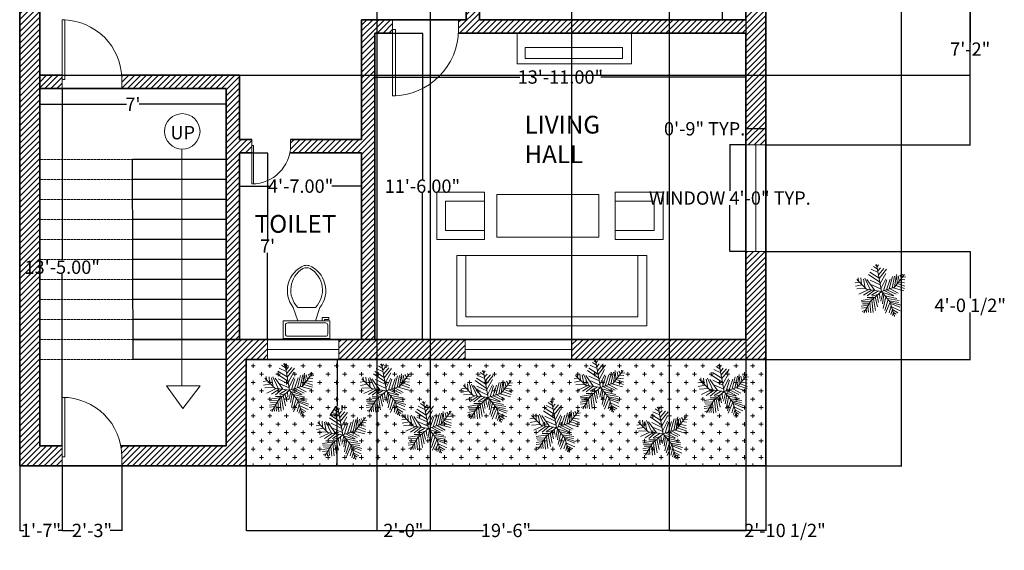
# Model space of a CAD drawing. Units: inches. Extents: x -20 to 887, y -143 to 410.
# Tile 4 of 5: x 443 to 887, y -143 to 96. Entities that reach past the tile are written whole.
import ezdxf

# ---------------------------------------------------------------- set-up
doc = ezdxf.new("R2010")
doc.units = ezdxf.units.IN
doc.header["$MEASUREMENT"] = 0
doc.linetypes.add('ACAD_ISO02W100', pattern=[15, 12, -3])
for name, color, linetype, lineweight in [('A-ANNO-DIMS', 2, 'Continuous', 18), ('A-ANNO-SYMB', 7, 'Continuous', 18), ('A-ANNO-TEXT', 7, 'Continuous', 18), ('A-AREA-IDEN', 7, 'Continuous', 25), ('A-DOOR', 3, 'Continuous', 18), ('A-FLOR-FIXT', 9, 'Continuous', 18), ('A-FLOR-STRS', 7, 'Continuous', 25), ('A-FLOR-STRS-OVHD', 8, 'ACAD_ISO02W100', 18), ('A-FURN', 8, 'Continuous', 18), ('A-GLAZ', 4, 'Continuous', 18), ('A-WALL', 7, 'Continuous', 35), ('A-WALL-PATT', 8, 'Continuous', 13), ('L-PLNT-PATT', 3, 'Continuous', 13), ('L-PLNT-TREE', 109, 'Continuous', 18)]:
    doc.layers.add(name, color=color, linetype=linetype, lineweight=lineweight)
doc.styles.get("Standard").update_dxf_attribs({"font": 'arial.ttf'})
doc.dimstyles.get("Standard").update_dxf_attribs({"dimtxt": 6, "dimasz": 0.18, "dimexe": 0.18, "dimexo": 0.0625, "dimgap": 0.09, "dimtad": 0, "dimtih": 1, "dimtoh": 1, "dimzin": 0, "dimdsep": 46, "dimlunit": 3, "dimtxsty": 'Standard', "dimcen": 0.09, "dimadec": 0, "dimazin": 0, "dimtfac": 1, "dimtofl": 0, "dimtmove": 0, "dimatfit": 3, "dimfxl": 1, "dimtolj": 1, "dimtzin": 0, "dimarcsym": 0})

# ---------------------------------------------------------------- blocks, each defined once
blk = doc.blocks.new('*U24')
for p, q in [((-7.288, 39.707), (-21.778, 46.673)), ((-8.737, 47.138), (-17.069, 52.711)), ((-10.186, 53.64), (-13.084, 55.962)), ((0, 0), (-10.5, 57)), ((-9.099, 51.782), (-6.563, 55.962)), ((-7.65, 43.423), (-2.578, 49.46)), ((-5.839, 35.992), (4.667, 48.067)), ((-5.114, 27.632), (10.463, 46.673)), ((-31.5, 4.5), (-52.5, 25.5)), ((-48.585, 21.131), (-49.309, 29.026)), ((-43.513, 28.561), (-42.427, 15.558)), ((-38.442, 26.239), (-34.819, 7.663)), ((-35.544, 28.097), (-24.314, 3.947)), ((-14.533, 2.09), (-30.834, 25.31)), ((-3.665, 19.273), (-27.574, 35.527)), ((-5.114, 28.097), (-24.676, 40.636)), ((-24.314, 23.917), (-2.941, 13.7)), ((-2.941, 16.486), (8.652, 37.85)), ((-1.129, 6.734), (9.014, 26.704)), ((3.942, 1.625), (11.187, 24.381)), ((10.101, 3.483), (17.708, 26.239)), ((16.259, 5.805), (23.142, 31.348)), ((22.055, 7.198), (27.489, 32.277)), ((27, 9), (48, 36)), ((27.127, 9.056), (31.112, 35.992)), ((31.836, 30.883), (32.561, 16.486)), ((35.096, 32.741), (37.27, 22.524)), ((38.719, 34.134), (41.979, 28.561)), ((40.53, 25.775), (48.862, 24.846)), ((43.791, 29.954), (51.036, 30.883)), ((44.153, 36.456), (45.239, 32.741)), ((-47.498, 19.737), (-55.83, 18.344)), ((-40.615, 13.7), (-55.105, 10.913)), ((-33.37, 6.269), (-52.207, 5.34)), ((-28.299, 3.483), (-47.86, -5.805)), ((-21.416, 3.018), (-38.079, -8.128)), ((0, 0), (-31.5, 4.5)), ((-15.982, 2.09), (-30.11, -9.521)), ((0, 0), (-22.5, -19.5)), ((-6.563, 1.161), (-21.416, -8.128)), ((-20.691, 13.7), (-1.129, 4.876)), ((0, 0), (27, 9)), ((0, 0), (18, -22.5)), ((6.478, 1.625), (26.04, -8.592)), ((11.187, 3.483), (30.749, -5.805)), ((18.07, 5.805), (35.096, -3.483)), ((24.229, 7.663), (46.688, 1.625)), ((29.662, 12.307), (48.137, 6.269)), ((33.285, 16.486), (48.862, 10.913)), ((36.183, 19.737), (48.137, 17.88)), ((-17.431, -15.094), (-42.789, -18.809)), ((-22.5, -19.5), (-37.5, -45)), ((-15.257, -12.772), (-30.11, -12.772)), ((-20.691, -18.345), (-17.793, -44.352)), ((-6.563, -5.805), (-19.967, -9.985)), ((-17.069, -15.094), (-12.721, -40.172)), ((-13.446, -11.378), (-8.737, -32.741)), ((-9.461, -8.592), (-6.201, -23.453)), ((-4.752, -3.483), (-3.665, -14.629)), ((2.493, -3.019), (-1.491, -20.202)), ((1.769, -2.555), (24.229, -9.521)), ((5.029, -6.27), (2.131, -25.775)), ((9.014, -11.378), (3.58, -35.992)), ((14.085, -16.951), (6.478, -40.172)), ((7.565, -9.056), (32.198, -14.629)), ((12.274, -15.094), (36.907, -18.809)), ((16.259, -19.738), (36.183, -22.989)), ((-28.299, -29.026), (-42.789, -31.348)), ((-24.314, -21.596), (-42.427, -22.06)), ((-30.834, -34.135), (-42.427, -35.528)), ((-34.457, -39.708), (-40.978, -42.494)), ((-26.849, -26.24), (-40.253, -25.775)), ((-32.646, -36.921), (-31.921, -44.352)), ((-29.023, -30.884), (-27.936, -43.887)), ((-25.038, -23.918), (-22.865, -45.281)), ((18.07, -22.524), (8.289, -45.745)), ((20.244, -30.419), (15.897, -44.816)), ((18, -22.5), (27, -52.5)), ((18.433, -22.524), (40.53, -29.026)), ((19.157, -25.311), (38.719, -33.206)), ((22.78, -37.85), (19.519, -48.532)), ((21.331, -32.741), (39.081, -40.636)), ((22.78, -38.314), (34.372, -44.816)), ((24.591, -45.745), (23.142, -50.854)), ((24.591, -43.423), (30.749, -47.603)), ((26.764, -49.925), (28.213, -50.854))]:
    blk.add_line(p, q)
blk = doc.blocks.new('*U2')
for p, q in [((0, 0), (0, -6)), ((40, 0), (40, -6))]:
    blk.add_line(p, q)
blk.add_lwpolyline([(0, 0), (0, 40), (1.75, 40), (1.75, 0)], close=True)
blk.add_arc((0, 0), 40, 0, 90)
blk = doc.blocks.new('*U6')
for p, q in [((9.5, -6), (9.5, -2)), ((-10, -8.5), (-8, -8.5)), ((-10, -9.5), (-10, -8.5)), ((-8, -8.5), (-8, -8)), ((-7, -8), (-7, -9.5)), ((-4, -8), (-6, -14)), ((4, -8), (6, -14)), ((-7, -9.5), (-10, -9.5)), ((4, -14), (-4, -14))]:
    blk.add_line(p, q)
blk.add_lwpolyline([(10.5, -8), (10.5, 0), (-10.5, 0), (-10.5, -8)], close=True)
for points in [[(-9.5, -2), (-9.5, -6)], [(8.5, -1), (-8.5, -1)], [(-8.5, -7), (8.5, -7)]]:
    blk.add_lwpolyline(points)
for centre, radius, start, end in [((-8.62, -1.88), 0.884, 81.8699, 188.1301), ((8.62, -1.88), 0.884, 351.8699, 98.1301), ((-8.62, -6.12), 0.884, 171.8699, 278.1301), ((8.62, -6.12), 0.884, 261.8699, 8.1301), ((3.52, -21.58), 12.17, 141.4691, 247.9714), ((4.2, -21.82), 11.33, 136.3677, 238.9468), ((-3.52, -21.58), 12.17, 292.0284, 38.5307), ((-4.2, -21.82), 11.33, 301.053, 43.6321), ((0, -27.88), 4, 245.7318, 294.2682), ((0, -29), 4, 254.8605, 285.1395)]:
    blk.add_arc(centre, radius, start, end)
blk = doc.blocks.new('*D26')
at = {"layer": 'A-ANNO-DIMS', "color": 0, "lineweight": -2, "transparency": 16777216}
for p, q in [((779.39, 374.92), (840.59, 374.92)), ((840.41, 374.74), (840.41, 138.07)), ((840.41, -104.9), (840.41, 131.76)), ((779.39, -105.08), (840.59, -105.08))]:
    blk.add_line(p, q, dxfattribs=at)
at = {"layer": 'A-ANNO-DIMS', "color": 0, "transparency": 16777216}
for points in [[(840.38, 374.74), (840.44, 374.74), (840.41, 374.92)], [(840.38, -104.9), (840.44, -104.9), (840.41, -105.08)]]:
    blk.add_solid(points, dxfattribs=at)
at = {"layer": 'Defpoints', "color": 0, "transparency": 16777216}
for p in [(779.33, 374.92), (779.33, -105.08), (840.41, -105.08)]:
    blk.add_point(p, dxfattribs=at)
at = {"layer": 'A-ANNO-DIMS', "color": 0, "transparency": 16777216, "insert": (840.41, 134.92), "char_height": 6, "attachment_point": 5}
blk.add_mtext("\\A1;40'", dxfattribs=at)
blk = doc.blocks.new('*D27')
at = {"layer": 'A-ANNO-DIMS', "color": 0, "lineweight": -2, "transparency": 16777216}
for p, q in [((586.94, -57.08), (586.06, -57.08)), ((586.24, -57.26), (586.24, -77.99)), ((586.24, -104.9), (586.24, -84.17)), ((586.94, -105.08), (586.06, -105.08))]:
    blk.add_line(p, q, dxfattribs=at)
at = {"layer": 'A-ANNO-DIMS', "color": 0, "transparency": 16777216}
for points in [[(586.21, -57.26), (586.27, -57.26), (586.24, -57.08)], [(586.21, -104.9), (586.27, -104.9), (586.24, -105.08)]]:
    blk.add_solid(points, dxfattribs=at)
at = {"layer": 'Defpoints', "color": 0, "transparency": 16777216}
for p in [(587.01, -57.08), (586.24, -105.08), (587.01, -105.08)]:
    blk.add_point(p, dxfattribs=at)
at = {"layer": 'A-ANNO-DIMS', "color": 0, "transparency": 16777216, "insert": (586.24, -81.08), "char_height": 6, "attachment_point": 5}
blk.add_mtext("\\A1;4'", dxfattribs=at)
blk = doc.blocks.new('*D28')
at = {"layer": 'A-ANNO-DIMS', "color": 0, "lineweight": -2, "transparency": 16777216}
for p, q in [((603.39, 89.92), (624.86, 89.92)), ((624.68, 89.74), (624.68, 24.07)), ((624.68, -47.9), (624.68, 17.76)), ((603.39, -48.08), (624.86, -48.08))]:
    blk.add_line(p, q, dxfattribs=at)
at = {"layer": 'A-ANNO-DIMS', "color": 0, "transparency": 16777216}
for points in [[(624.65, 89.74), (624.71, 89.74), (624.68, 89.92)], [(624.65, -47.9), (624.71, -47.9), (624.68, -48.08)]]:
    blk.add_solid(points, dxfattribs=at)
at = {"layer": 'Defpoints', "color": 0, "transparency": 16777216}
for p in [(603.33, 89.92), (603.33, -48.08), (624.68, -48.08)]:
    blk.add_point(p, dxfattribs=at)
at = {"layer": 'A-ANNO-DIMS', "color": 0, "transparency": 16777216, "insert": (624.68, 20.92), "char_height": 6, "attachment_point": 5}
blk.add_mtext('\\A1;11\'-6.00"', dxfattribs=at)
blk = doc.blocks.new('*D29')
at = {"layer": 'A-ANNO-DIMS', "color": 0, "lineweight": -2, "transparency": 16777216}
for p, q in [((603.33, 89.86), (603.33, 69.91)), ((770.33, 89.86), (770.33, 69.91)), ((603.51, 70.09), (668.56, 70.09)), ((770.15, 70.09), (705.1, 70.09))]:
    blk.add_line(p, q, dxfattribs=at)
at = {"layer": 'A-ANNO-DIMS', "color": 0, "transparency": 16777216}
for points in [[(603.51, 70.12), (603.51, 70.06), (603.33, 70.09)], [(770.15, 70.12), (770.15, 70.06), (770.33, 70.09)]]:
    blk.add_solid(points, dxfattribs=at)
at = {"layer": 'Defpoints', "color": 0, "transparency": 16777216}
for p in [(603.33, 89.92), (770.33, 89.92), (770.33, 70.09)]:
    blk.add_point(p, dxfattribs=at)
at = {"layer": 'A-ANNO-DIMS', "color": 0, "transparency": 16777216, "insert": (686.83, 70.09), "char_height": 6, "attachment_point": 5}
blk.add_mtext('\\A1;13\'-11.00"', dxfattribs=at)
blk = doc.blocks.new('*D30')
at = {"layer": 'A-ANNO-DIMS', "color": 0, "lineweight": -2, "transparency": 16777216}
for p, q in [((545.19, 35.92), (555.12, 35.92)), ((554.94, 35.74), (554.94, -2.99)), ((554.94, -47.9), (554.94, -9.17)), ((542.39, -48.08), (555.12, -48.08))]:
    blk.add_line(p, q, dxfattribs=at)
at = {"layer": 'A-ANNO-DIMS', "color": 0, "transparency": 16777216}
for points in [[(554.91, 35.74), (554.97, 35.74), (554.94, 35.92)], [(554.91, -47.9), (554.97, -47.9), (554.94, -48.08)]]:
    blk.add_solid(points, dxfattribs=at)
at = {"layer": 'Defpoints', "color": 0, "transparency": 16777216}
for p in [(545.13, 35.92), (542.33, -48.08), (554.94, -48.08)]:
    blk.add_point(p, dxfattribs=at)
at = {"layer": 'A-ANNO-DIMS', "color": 0, "transparency": 16777216, "insert": (554.94, -6.08), "char_height": 6, "attachment_point": 5}
blk.add_mtext("\\A1;7'", dxfattribs=at)
blk = doc.blocks.new('*D31')
at = {"layer": 'A-ANNO-DIMS', "color": 0, "lineweight": -2, "transparency": 16777216}
for p, q in [((542.33, 35.86), (542.33, 20.76)), ((597.33, 35.86), (597.33, 20.76)), ((542.51, 20.94), (555.82, 20.94)), ((597.15, 20.94), (583.84, 20.94))]:
    blk.add_line(p, q, dxfattribs=at)
at = {"layer": 'A-ANNO-DIMS', "color": 0, "transparency": 16777216}
for points in [[(542.51, 20.97), (542.51, 20.91), (542.33, 20.94)], [(597.15, 20.97), (597.15, 20.91), (597.33, 20.94)]]:
    blk.add_solid(points, dxfattribs=at)
at = {"layer": 'Defpoints', "color": 0, "transparency": 16777216}
for p in [(542.33, 35.92), (597.33, 35.92), (597.33, 20.94)]:
    blk.add_point(p, dxfattribs=at)
at = {"layer": 'A-ANNO-DIMS', "color": 0, "transparency": 16777216, "insert": (569.83, 20.94), "char_height": 6, "attachment_point": 5}
blk.add_mtext('\\A1;4\'-7.00"', dxfattribs=at)
blk = doc.blocks.new('*D32')
at = {"layer": 'A-ANNO-DIMS', "color": 0, "lineweight": -2, "transparency": 16777216}
for p, q in [((452.39, 64.92), (462.66, 64.92)), ((462.48, 64.74), (462.48, -12.43)), ((462.48, -95.9), (462.48, -18.74)), ((452.39, -96.08), (462.66, -96.08))]:
    blk.add_line(p, q, dxfattribs=at)
at = {"layer": 'A-ANNO-DIMS', "color": 0, "transparency": 16777216}
for points in [[(462.45, 64.74), (462.51, 64.74), (462.48, 64.92)], [(462.45, -95.9), (462.51, -95.9), (462.48, -96.08)]]:
    blk.add_solid(points, dxfattribs=at)
at = {"layer": 'Defpoints', "color": 0, "transparency": 16777216}
for p in [(452.33, 64.92), (462.48, 64.92), (452.33, -96.08)]:
    blk.add_point(p, dxfattribs=at)
at = {"layer": 'A-ANNO-DIMS', "color": 0, "transparency": 16777216, "insert": (462.48, -15.58), "char_height": 6, "attachment_point": 5}
blk.add_mtext('\\A1;13\'-5.00"', dxfattribs=at)
blk = doc.blocks.new('*D33')
at = {"layer": 'A-ANNO-DIMS', "color": 0, "lineweight": -2, "transparency": 16777216}
for p, q in [((452.33, 64.86), (452.33, 57.63)), ((536.33, 64.86), (536.33, 57.63)), ((452.51, 57.81), (491.5, 57.81)), ((536.15, 57.81), (497.15, 57.81))]:
    blk.add_line(p, q, dxfattribs=at)
at = {"layer": 'A-ANNO-DIMS', "color": 0, "transparency": 16777216}
for points in [[(452.51, 57.84), (452.51, 57.78), (452.33, 57.81)], [(536.15, 57.84), (536.15, 57.78), (536.33, 57.81)]]:
    blk.add_solid(points, dxfattribs=at)
at = {"layer": 'Defpoints', "color": 0, "transparency": 16777216}
for p in [(452.33, 64.92), (536.33, 64.92), (536.33, 57.81)]:
    blk.add_point(p, dxfattribs=at)
at = {"layer": 'A-ANNO-DIMS', "color": 0, "transparency": 16777216, "insert": (494.33, 57.81), "char_height": 6, "attachment_point": 5}
blk.add_mtext("\\A1;7'", dxfattribs=at)
blk = doc.blocks.new('*D34')
at = {"layer": 'A-ANNO-DIMS', "color": 0, "lineweight": -2, "transparency": 16777216}
for p, q in [((770.27, 215.92), (759.59, 215.92)), ((759.77, 215.74), (759.77, 159.07)), ((759.77, 96.1), (759.77, 152.76)), ((770.27, 95.92), (759.59, 95.92))]:
    blk.add_line(p, q, dxfattribs=at)
at = {"layer": 'A-ANNO-DIMS', "color": 0, "transparency": 16777216}
for points in [[(759.74, 215.74), (759.8, 215.74), (759.77, 215.92)], [(759.74, 96.1), (759.8, 96.1), (759.77, 95.92)]]:
    blk.add_solid(points, dxfattribs=at)
at = {"layer": 'Defpoints', "color": 0, "transparency": 16777216}
for p in [(770.33, 215.92), (759.77, 95.92), (770.33, 95.92)]:
    blk.add_point(p, dxfattribs=at)
at = {"layer": 'A-ANNO-DIMS', "color": 0, "transparency": 16777216, "insert": (759.77, 155.92), "char_height": 6, "attachment_point": 5}
blk.add_mtext("\\A1;10'", dxfattribs=at)
blk = doc.blocks.new('WIN-48IN-9IN-WALL')
for p, q in [((9, 48), (0, 48)), ((4.5, 0), (4.5, 48)), ((9, 0), (0, 0))]:
    blk.add_line(p, q)
blk = doc.blocks.new('*D43')
at = {"layer": 'A-ANNO-DIMS', "color": 0, "lineweight": -2, "transparency": 16777216}
for p, q in [((770.27, 39.57), (762.95, 39.57)), ((763.13, 39.39), (763.13, 18.77)), ((763.13, -8.25), (763.13, 12.38)), ((770.27, -8.43), (762.95, -8.43))]:
    blk.add_line(p, q, dxfattribs=at)
at = {"layer": 'A-ANNO-DIMS', "color": 0, "transparency": 16777216}
for points in [[(763.1, 39.39), (763.16, 39.39), (763.13, 39.57)], [(763.1, -8.25), (763.16, -8.25), (763.13, -8.43)]]:
    blk.add_solid(points, dxfattribs=at)
at = {"layer": 'Defpoints', "color": 0, "transparency": 16777216}
for p in [(770.33, 39.57), (763.13, -8.43), (770.33, -8.43)]:
    blk.add_point(p, dxfattribs=at)
at = {"layer": 'A-ANNO-DIMS', "color": 0, "transparency": 16777216, "insert": (763.13, 15.57), "char_height": 6, "attachment_point": 5}
blk.add_mtext('\\A1;WINDOW 4\'-0" TYP.', dxfattribs=at)
blk = doc.blocks.new('*D44')
at = {"layer": 'A-ANNO-DIMS', "color": 0, "lineweight": -2, "transparency": 16777216}
for p, q in [((770.33, 46.77), (770.15, 46.77)), ((770.33, 39.64), (770.33, 46.95)), ((779.15, 46.77), (770.51, 46.77)), ((779.33, 39.64), (779.33, 46.95))]:
    blk.add_line(p, q, dxfattribs=at)
at = {"layer": 'A-ANNO-DIMS', "color": 0, "transparency": 16777216}
for points in [[(770.51, 46.8), (770.51, 46.74), (770.33, 46.77)], [(779.15, 46.8), (779.15, 46.74), (779.33, 46.77)]]:
    blk.add_solid(points, dxfattribs=at)
at = {"layer": 'Defpoints', "color": 0, "transparency": 16777216}
for p in [(770.33, 46.77), (770.33, 39.57), (779.33, 39.57)]:
    blk.add_point(p, dxfattribs=at)
at = {"layer": 'A-ANNO-DIMS', "color": 0, "transparency": 16777216, "insert": (751.77, 46.77), "char_height": 6, "attachment_point": 5}
blk.add_mtext('\\A1;0\'-9" TYP.', dxfattribs=at)
blk = doc.blocks.new('*D45')
at = {"layer": 'A-ANNO-DIMS', "color": 0, "lineweight": -2, "transparency": 16777216}
for p, q in [((690.33, 116.26), (690.33, 104.14)), ((770.33, 116.26), (770.33, 104.14)), ((690.51, 104.32), (770.15, 104.32)), ((770.33, 104.32), (770.51, 104.32))]:
    blk.add_line(p, q, dxfattribs=at)
at = {"layer": 'A-ANNO-DIMS', "color": 0, "transparency": 16777216}
for points in [[(690.51, 104.35), (690.51, 104.29), (690.33, 104.32)], [(770.15, 104.35), (770.15, 104.29), (770.33, 104.32)]]:
    blk.add_solid(points, dxfattribs=at)
at = {"layer": 'Defpoints', "color": 0, "transparency": 16777216}
for p in [(690.33, 116.32), (770.33, 116.32), (770.33, 104.32)]:
    blk.add_point(p, dxfattribs=at)
at = {"layer": 'A-ANNO-DIMS', "color": 0, "transparency": 16777216, "insert": (814.73, 104.32), "char_height": 6, "attachment_point": 5}
blk.add_mtext('\\A1;QUEEN BED 6\'-8" TYP.', dxfattribs=at)
blk = doc.blocks.new('*D72')
at = {"layer": 'A-ANNO-DIMS', "color": 0, "lineweight": -2, "transparency": 16777216}
for p, q in [((443.33, -105.14), (443.33, -134.33)), ((462.48, -105.14), (462.48, -134.33)), ((443.51, -134.15), (445.12, -134.15)), ((462.3, -134.15), (460.69, -134.15))]:
    blk.add_line(p, q, dxfattribs=at)
at = {"layer": 'A-ANNO-DIMS', "color": 0, "transparency": 16777216}
for points in [[(443.51, -134.12), (443.51, -134.18), (443.33, -134.15)], [(462.3, -134.12), (462.3, -134.18), (462.48, -134.15)]]:
    blk.add_solid(points, dxfattribs=at)
at = {"layer": 'Defpoints', "color": 0, "transparency": 16777216}
for p in [(443.33, -105.08), (462.48, -105.08), (462.48, -134.15)]:
    blk.add_point(p, dxfattribs=at)
at = {"layer": 'A-ANNO-DIMS', "color": 0, "transparency": 16777216, "insert": (452.91, -134.15), "char_height": 6, "attachment_point": 5}
blk.add_mtext('\\A1;1\'-7"', dxfattribs=at)
blk = doc.blocks.new('*D73')
at = {"layer": 'A-ANNO-DIMS', "color": 0, "lineweight": -2, "transparency": 16777216}
for p, q in [((462.48, -105.14), (462.48, -134.33)), ((489.34, -105.14), (489.34, -134.33)), ((462.66, -134.15), (467.8, -134.15)), ((489.16, -134.15), (484.03, -134.15))]:
    blk.add_line(p, q, dxfattribs=at)
at = {"layer": 'A-ANNO-DIMS', "color": 0, "transparency": 16777216}
for points in [[(462.66, -134.12), (462.66, -134.18), (462.48, -134.15)], [(489.16, -134.12), (489.16, -134.18), (489.34, -134.15)]]:
    blk.add_solid(points, dxfattribs=at)
at = {"layer": 'Defpoints', "color": 0, "transparency": 16777216}
for p in [(462.48, -105.08), (489.34, -105.08), (489.34, -134.15)]:
    blk.add_point(p, dxfattribs=at)
at = {"layer": 'A-ANNO-DIMS', "color": 0, "transparency": 16777216, "insert": (475.91, -134.15), "char_height": 6, "attachment_point": 5}
blk.add_mtext('\\A1;2\'-3"', dxfattribs=at)
blk = doc.blocks.new('*D74')
at = {"layer": 'A-ANNO-DIMS', "color": 0, "lineweight": -2, "transparency": 16777216}
for p, q in [((545.33, -105.14), (545.33, -134.33)), ((779.33, -105.14), (779.33, -134.33)), ((545.51, -134.15), (652.21, -134.15)), ((779.15, -134.15), (672.44, -134.15))]:
    blk.add_line(p, q, dxfattribs=at)
at = {"layer": 'A-ANNO-DIMS', "color": 0, "transparency": 16777216}
for points in [[(545.51, -134.12), (545.51, -134.18), (545.33, -134.15)], [(779.15, -134.12), (779.15, -134.18), (779.33, -134.15)]]:
    blk.add_solid(points, dxfattribs=at)
at = {"layer": 'Defpoints', "color": 0, "transparency": 16777216}
for p in [(545.33, -105.08), (779.33, -105.08), (779.33, -134.15)]:
    blk.add_point(p, dxfattribs=at)
at = {"layer": 'A-ANNO-DIMS', "color": 0, "transparency": 16777216, "insert": (662.33, -134.15), "char_height": 6, "attachment_point": 5}
blk.add_mtext('\\A1;19\'-6"', dxfattribs=at)
blk = doc.blocks.new('*D75')
at = {"layer": 'A-ANNO-DIMS', "color": 0, "lineweight": -2, "transparency": 16777216}
for p, q in [((692.01, -57.02), (692.01, 401.55)), ((692.19, 401.37), (720.64, 401.37)), ((779.15, 401.37), (750.7, 401.37)), ((779.33, -57.02), (779.33, 401.55))]:
    blk.add_line(p, q, dxfattribs=at)
at = {"layer": 'A-ANNO-DIMS', "color": 0, "transparency": 16777216}
for points in [[(692.19, 401.4), (692.19, 401.34), (692.01, 401.37)], [(779.15, 401.4), (779.15, 401.34), (779.33, 401.37)]]:
    blk.add_solid(points, dxfattribs=at)
at = {"layer": 'Defpoints', "color": 0, "transparency": 16777216}
for p in [(779.33, 401.37), (692.01, -57.08), (779.33, -57.08)]:
    blk.add_point(p, dxfattribs=at)
at = {"layer": 'A-ANNO-DIMS', "color": 0, "transparency": 16777216, "insert": (735.67, 401.37), "char_height": 6, "attachment_point": 5}
blk.add_mtext('\\A1;7\'-3 1/2"', dxfattribs=at)
blk = doc.blocks.new('*D76')
at = {"layer": 'A-ANNO-DIMS', "color": 0, "lineweight": -2, "transparency": 16777216}
for p, q in [((779.39, -8.43), (871.56, -8.43)), ((871.38, -8.61), (871.38, -29.56)), ((871.38, -56.9), (871.38, -35.95)), ((779.39, -57.08), (871.56, -57.08))]:
    blk.add_line(p, q, dxfattribs=at)
at = {"layer": 'A-ANNO-DIMS', "color": 0, "transparency": 16777216}
for points in [[(871.35, -8.61), (871.41, -8.61), (871.38, -8.43)], [(871.35, -56.9), (871.41, -56.9), (871.38, -57.08)]]:
    blk.add_solid(points, dxfattribs=at)
at = {"layer": 'Defpoints', "color": 0, "transparency": 16777216}
for p in [(779.33, -8.43), (871.38, -8.43), (779.33, -57.08)]:
    blk.add_point(p, dxfattribs=at)
at = {"layer": 'A-ANNO-DIMS', "color": 0, "transparency": 16777216, "insert": (871.38, -32.75), "char_height": 6, "attachment_point": 5}
blk.add_mtext('\\A1;4\'-0 1/2"', dxfattribs=at)
blk = doc.blocks.new('*D77')
at = {"layer": 'A-ANNO-DIMS', "color": 0, "lineweight": -2, "transparency": 16777216}
for p, q in [((779.39, 125.72), (871.56, 125.72)), ((871.38, 125.54), (871.38, 85.75)), ((871.38, 39.75), (871.38, 79.55)), ((779.39, 39.57), (871.56, 39.57))]:
    blk.add_line(p, q, dxfattribs=at)
at = {"layer": 'A-ANNO-DIMS', "color": 0, "transparency": 16777216}
for points in [[(871.35, 125.54), (871.41, 125.54), (871.38, 125.72)], [(871.35, 39.75), (871.41, 39.75), (871.38, 39.57)]]:
    blk.add_solid(points, dxfattribs=at)
at = {"layer": 'Defpoints', "color": 0, "transparency": 16777216}
for p in [(779.33, 125.72), (871.38, 125.72), (779.33, 39.57)]:
    blk.add_point(p, dxfattribs=at)
at = {"layer": 'A-ANNO-DIMS', "color": 0, "transparency": 16777216, "insert": (871.38, 82.65), "char_height": 6, "attachment_point": 5}
blk.add_mtext('\\A1;7\'-2"', dxfattribs=at)
blk = doc.blocks.new('*D79')
at = {"layer": 'A-ANNO-DIMS', "color": 0, "lineweight": -2, "transparency": 16777216}
for p, q in [((735.77, 365.86), (735.77, -134.33)), ((770.33, 365.86), (770.33, -134.33)), ((735.95, -134.15), (770.15, -134.15)), ((770.33, -134.15), (770.51, -134.15))]:
    blk.add_line(p, q, dxfattribs=at)
at = {"layer": 'A-ANNO-DIMS', "color": 0, "transparency": 16777216}
for points in [[(735.95, -134.12), (735.95, -134.18), (735.77, -134.15)], [(770.15, -134.12), (770.15, -134.18), (770.33, -134.15)]]:
    blk.add_solid(points, dxfattribs=at)
at = {"layer": 'Defpoints', "color": 0, "transparency": 16777216}
for p in [(735.77, 365.92), (770.33, 365.92), (770.33, -134.15)]:
    blk.add_point(p, dxfattribs=at)
at = {"layer": 'A-ANNO-DIMS', "color": 0, "transparency": 16777216, "insert": (787.95, -134.15), "char_height": 6, "attachment_point": 5}
blk.add_mtext('\\A1;2\'-10 1/2"', dxfattribs=at)
blk = doc.blocks.new('*D81')
at = {"layer": 'A-ANNO-DIMS', "color": 0, "lineweight": -2, "transparency": 16777216}
for p, q in [((604.12, 365.86), (604.12, -134.33)), ((628.12, 365.86), (628.12, -134.33)), ((604.3, -134.15), (608.01, -134.15)), ((627.94, -134.15), (624.24, -134.15))]:
    blk.add_line(p, q, dxfattribs=at)
at = {"layer": 'A-ANNO-DIMS', "color": 0, "transparency": 16777216}
for points in [[(604.3, -134.12), (604.3, -134.18), (604.12, -134.15)], [(627.94, -134.12), (627.94, -134.18), (628.12, -134.15)]]:
    blk.add_solid(points, dxfattribs=at)
at = {"layer": 'Defpoints', "color": 0, "transparency": 16777216}
for p in [(604.12, 365.92), (628.12, 365.92), (628.12, -134.15)]:
    blk.add_point(p, dxfattribs=at)
at = {"layer": 'A-ANNO-DIMS', "color": 0, "transparency": 16777216, "insert": (616.12, -134.15), "char_height": 6, "attachment_point": 5}
blk.add_mtext('\\A1;2\'-0"', dxfattribs=at)
blk = doc.blocks.new('*D85')
at = {"layer": 'A-ANNO-DIMS', "color": 0, "lineweight": -2, "transparency": 16777216}
for p, q in [((452.39, 215.92), (871.56, 215.92)), ((871.38, 215.74), (871.38, 146.52)), ((871.38, 71.1), (871.38, 140.32)), ((452.39, 70.92), (871.56, 70.92))]:
    blk.add_line(p, q, dxfattribs=at)
at = {"layer": 'A-ANNO-DIMS', "color": 0, "transparency": 16777216}
for points in [[(871.35, 215.74), (871.41, 215.74), (871.38, 215.92)], [(871.35, 71.1), (871.41, 71.1), (871.38, 70.92)]]:
    blk.add_solid(points, dxfattribs=at)
at = {"layer": 'Defpoints', "color": 0, "transparency": 16777216}
for p in [(452.33, 215.92), (452.33, 70.92), (871.38, 70.92)]:
    blk.add_point(p, dxfattribs=at)
at = {"layer": 'A-ANNO-DIMS', "color": 0, "transparency": 16777216, "insert": (871.38, 143.42), "char_height": 6, "attachment_point": 5}
blk.add_mtext('\\A1;12\'-1"', dxfattribs=at)

msp = doc.modelspace()

# ---------------------------------------------------------------- hatches: boundary and pattern name
at = {"layer": 'A-WALL-PATT'}
h = msp.add_hatch(dxfattribs=at)
h.set_pattern_fill('ANSI31', color=256, scale=15)
h.paths.add_polyline_path([(779.328, 125.723), (770.328, 125.723), (770.328, 116.321), (770.328, 95.918), (650.328, 95.918), (650.328, 109.352), (648.356, 109.352), (644.328, 109.352), (644.328, 95.918), (640.97, 95.918), (640.97, 91.453, -0.0129025), (640.93, 89.918), (770.328, 89.918), (770.328, 39.573), (779.328, 39.573)])
h.paths.add_polyline_path([(779.328, -8.427), (770.328, -8.427), (770.328, -48.082), (692.012, -48.082), (692.012, -57.082), (779.328, -57.082)])
h.paths.add_polyline_path([(644.012, -48.082), (587.007, -48.082), (587.007, -57.082), (644.012, -57.082)])
h.paths.add_polyline_path([(603.328, 89.918), (611.206, 89.918), (611.206, 91.453), (611.206, 95.918), (597.328, 95.918), (597.328, 41.918), (565.317, 41.918), (565.317, 39.309, -0.049098), (564.984, 35.918), (597.328, 35.918), (597.328, -48.082), (603.328, -48.082)])
h.paths.add_polyline_path([(545.328, -57.082), (554.942, -57.082), (554.942, -48.082), (536.328, -48.082), (536.328, -96.082), (488.875, -96.082, -0.0465845), (489.339, -101.054), (489.339, -105.082), (545.328, -105.082)])
h.paths.add_polyline_path([(452.328, 103.65), (443.328, 103.65), (443.328, -105.082), (462.484, -105.082), (462.484, -101.054), (462.484, -96.082), (452.328, -96.082)])
h = msp.add_hatch(dxfattribs=at)
h.set_pattern_fill('ANSI31', color=256, scale=15)
h.paths.add_polyline_path([(462.484, 68.994), (462.484, 70.918), (452.328, 70.918), (452.328, 64.918), (462.484, 64.918)])
h = msp.add_hatch(dxfattribs=at)
h.set_pattern_fill('ANSI31', color=256, scale=15)
h.paths.add_polyline_path([(542.328, 70.918), (489.27, 70.918, -0.0179288), (489.339, 68.994), (489.339, 64.918), (536.328, 64.918), (536.328, -48.082), (542.328, -48.082), (542.328, 35.918), (547.925, 35.918), (547.925, 39.309), (547.925, 41.918), (542.328, 41.918)])
at = {"layer": 'L-PLNT-PATT'}
h = msp.add_hatch(dxfattribs=at)
h.set_pattern_fill('CROSS', color=256, scale=15)
h.paths.add_polyline_path([(779.328, -57.082), (545.328, -57.082), (545.328, -105.082), (779.328, -105.082)])

# ---------------------------------------------------------------- linework, layer by layer
at = {"layer": 'A-ANNO-SYMB'}
for p, q in [((516.396, -57.082), (516.396, 37.645)), ((516.396, -57.082), (516.396, -68.982)), ((516.396, -68.982), (509.496, -68.982)), ((509.496, -68.982), (516.802, -79.277)), ((516.396, -68.982), (524.669, -68.982)), ((516.802, -79.277), (524.669, -68.982))]:
    msp.add_line(p, q, dxfattribs=at)
msp.add_circle((516.56, 45.62), 7.977, dxfattribs=at)
at = {"layer": 'A-FLOR-STRS'}
msp.add_line((494.39, -57.082), (494.078, 32.918), dxfattribs=at)
for points in [[(536.328, 32.918), (494.078, 32.918)], [(536.328, 23.918), (494.109, 23.918)], [(536.328, 14.918), (494.14, 14.918)], [(536.328, 5.918), (494.171, 5.918)], [(536.328, -3.082), (494.203, -3.082)], [(536.328, -12.082), (494.234, -12.082)], [(536.328, -21.082), (494.265, -21.082)], [(536.328, -30.082), (494.297, -30.082)], [(536.328, -39.082), (494.328, -39.082)], [(536.328, -57.082), (494.39, -57.082)]]:
    msp.add_lwpolyline(points, dxfattribs=at)
at = {"layer": 'A-FLOR-STRS-OVHD', "ltscale": 0.1}
for p, q in [((494.39, 32.918), (452.328, 32.918)), ((494.39, 23.918), (452.328, 23.918)), ((494.39, 14.918), (452.328, 14.918)), ((494.39, 5.918), (452.328, 5.918)), ((494.39, -3.082), (452.328, -3.082)), ((494.39, -12.082), (452.328, -12.082)), ((494.39, -21.082), (452.328, -21.082)), ((494.39, -30.082), (452.328, -30.082)), ((494.39, -39.082), (452.328, -39.082)), ((494.39, -48.082), (452.328, -48.082)), ((494.39, -57.082), (452.328, -57.082))]:
    msp.add_line(p, q, dxfattribs=at)
at = {"layer": 'A-FURN'}
for points in [[(667.304, 89.918), (718.818, 89.918), (718.818, 75.959), (667.304, 75.959)], [(671.03, 83.407), (714.872, 83.407), (714.872, 78.368), (671.03, 78.368)], [(631.147, 18.173), (652.709, 18.173), (652.709, -3.026), (631.147, -3.026)], [(711.482, 18.173), (733.043, 18.173), (733.043, -3.026), (711.482, -3.026)], [(658.273, 17.13), (704.178, 17.13), (704.178, -1.984), (658.273, -1.984)], [(640.189, -10.324), (725.74, -10.324), (725.74, -41.949), (640.189, -41.949)]]:
    msp.add_lwpolyline(points, close=True, dxfattribs=at)
for points in [[(652.709, 0.974), (635.147, 0.974), (635.147, 14.173), (652.709, 14.173)], [(711.482, 14.173), (729.043, 14.173), (729.043, 0.974), (711.482, 0.974)], [(721.74, -10.324), (721.74, -37.949), (644.189, -37.949), (644.189, -10.324)]]:
    msp.add_lwpolyline(points, dxfattribs=at)
at = {"layer": 'A-GLAZ'}
for p, q in [((554.942, -48.082), (554.942, -57.082)), ((587.007, -48.082), (587.007, -57.082)), ((554.942, -52.582), (587.007, -52.582))]:
    msp.add_line(p, q, dxfattribs=at)
at = {"layer": 'A-WALL'}
for points in [[(443.328, 374.918), (779.328, 374.918), (779.328, -105.082)], [(443.328, -105.082), (443.328, 374.918)], [(452.328, -96.082), (452.328, 365.918)], [(770.328, 365.918), (770.328, 95.918)], [(644.328, 109.352), (644.328, 95.918)], [(650.328, 109.352), (650.328, 95.918)], [(597.328, 95.918), (597.328, 41.918)], [(644.328, 95.918), (597.328, 95.918)], [(770.328, 95.918), (650.328, 95.918)], [(603.328, 89.918), (603.328, -48.082)], [(611.206, 89.918), (603.328, 89.918)], [(770.328, 89.918), (640.93, 89.918)], [(770.328, 89.918), (770.328, -48.082)], [(462.484, 70.918), (452.328, 70.918)], [(542.328, 70.918), (489.27, 70.918)], [(542.328, 41.918), (542.328, 70.918)], [(536.328, 64.918), (452.328, 64.918)], [(536.328, -96.082), (536.328, 64.918)], [(547.925, 41.918), (542.328, 41.918)], [(597.328, 41.918), (565.317, 41.918)], [(542.328, -48.082), (542.328, 35.918)], [(547.925, 35.918), (542.328, 35.918)], [(597.328, 35.918), (564.984, 35.918)], [(597.328, 35.918), (597.328, -48.082)], [(770.328, -48.082), (494.359, -48.082)], [(779.328, -57.082), (545.328, -57.082)], [(545.328, -105.082), (545.328, -57.082)], [(462.484, -96.082), (452.328, -96.082)], [(536.328, -96.082), (488.875, -96.082)], [(779.328, -105.082), (443.328, -105.082)]]:
    msp.add_lwpolyline(points, dxfattribs=at)

# ---------------------------------------------------------------- block references
at = {"layer": 'A-DOOR', "xscale": 0.6713823920216754, "yscale": 0.6713823920216754, "zscale": 0.6713823920216754}
for p in [(462.484, 68.994), (462.484, -101.054)]:
    msp.add_blockref('*U2', p, dxfattribs=at)
at = {"layer": 'A-DOOR', "rotation": 180}
for p, xscale, yscale, zscale in [((611.206, 91.453), -0.7441059094740626, 0.7441059094740626, 0.7441059094740626), ((547.925, 39.309), -0.4348113241361661, 0.4348113241361661, 0.4348113241361661)]:
    msp.add_blockref('*U2', p, dxfattribs=dict(at, xscale=xscale, yscale=yscale, zscale=zscale))
at = {"layer": 'A-FLOR-FIXT', "rotation": 180}
msp.add_blockref('*U6', (572.539, -47.701), dxfattribs=at)
at = {"layer": 'A-GLAZ'}
for p, rotation in [((779.328, 39.574), 180), ((692.012, -57.082), 89.99999999999994)]:
    msp.add_blockref('WIN-48IN-9IN-WALL', p, dxfattribs=dict(at, rotation=rotation))
at = {"layer": 'L-PLNT-TREE', "xscale": 0.2136772059356402, "yscale": 0.2136772059356402, "zscale": 0.2136772059356402}
for p in [(831.482, -26.497), (704.887, -69.736), (564.902, -71.012), (608.564, -71.245), (654.338, -74.257), (760.644, -71.618), (588.785, -91.012), (627.401, -88.188), (685.042, -87.811), (733.142, -90.632)]:
    msp.add_blockref('*U24', p, dxfattribs=at)

# ---------------------------------------------------------------- texts
at = {"layer": 'A-ANNO-TEXT', "insert": (511.198, 48.041), "char_height": 6, "attachment_point": 1}
msp.add_mtext_dynamic_manual_height_columns('UP ', width=6.08345, gutter_width=1, heights=[0], dxfattribs=at)
at = {"layer": 'A-AREA-IDEN', "char_height": 8, "attachment_point": 1}
for s, insert in [('LIVING HALL', (670.665, 52.633)), ('TOILET', (549.171, 7.957))]:
    msp.add_mtext_dynamic_manual_height_columns(s, width=50.36765, gutter_width=1, heights=[0], dxfattribs=dict(at, insert=insert))

# ---------------------------------------------------------------- dimensions: what is measured, and where the dimension line sits
at = {"layer": 'A-ANNO-DIMS'}
for base, p1, p2, override, picture, middle in [((779.328, 401.368), (692.012, -57.082), (779.328, -57.082), {"dimdec": 1, "dimlfac": 1, "dimrnd": 0, "dimzin": 1, "dimdsep": 46, "dimlunit": 4, "dimfrac": 2}, '*D75', (735.67, 401.368)), ((628.122, -134.151), (604.122, 365.918), (628.122, 365.918), {"dimdec": 1, "dimlfac": 1, "dimrnd": 0, "dimzin": 1, "dimdsep": 46, "dimlunit": 4, "dimfrac": 2}, '*D81', (616.122, -134.151)), ((770.328, -134.151), (735.77, 365.918), (770.328, 365.918), {"dimdec": 1, "dimlfac": 1, "dimrnd": 0, "dimzin": 1, "dimdsep": 46, "dimlunit": 4, "dimfrac": 2}, '*D79', (787.945, -134.151)), ((770.328, 70.088), (603.328, 89.918), (770.328, 89.918), {"dimclrd": 0, "dimclre": 0, "dimclrt": 0}, '*D29', (686.828, 70.088)), ((536.328, 57.81), (452.328, 64.918), (536.328, 64.918), {"dimclrd": 0, "dimclre": 0, "dimclrt": 0}, '*D33', (494.328, 57.81)), ((597.328, 20.938), (542.328, 35.918), (597.328, 35.918), {"dimclrd": 0, "dimclre": 0, "dimclrt": 0}, '*D31', (569.828, 20.938)), ((462.484, -134.151), (443.328, -105.082), (462.484, -105.082), {"dimdec": 1, "dimlfac": 1, "dimrnd": 0, "dimzin": 1, "dimdsep": 46, "dimlunit": 4, "dimfrac": 2}, '*D72', (452.906, -134.151)), ((489.339, -134.151), (462.484, -105.082), (489.339, -105.082), {"dimdec": 1, "dimlfac": 1, "dimrnd": 0, "dimzin": 1, "dimdsep": 46, "dimlunit": 4, "dimfrac": 2}, '*D73', (475.912, -134.151)), ((779.328, -134.151), (545.328, -105.082), (779.328, -105.082), {"dimdec": 1, "dimlfac": 1, "dimrnd": 0, "dimzin": 1, "dimdsep": 46, "dimlunit": 4, "dimfrac": 2}, '*D74', (662.328, -134.151))]:
    dim = msp.add_linear_dim(base=base, p1=p1, p2=p2, dimstyle='Standard', override=override, dxfattribs=at)
    dim.commit()
    dim.dimension.update_dxf_attribs({"geometry": picture, "text_midpoint": middle})
for base, p1, p2, override, picture, middle in [((840.41, -105.082), (779.328, 374.918), (779.328, -105.082), {"dimclrd": 0, "dimclre": 0, "dimclrt": 0}, '*D26', (840.41, 134.918)), ((871.381, 70.918), (452.328, 215.918), (452.328, 70.918), {"dimdec": 1, "dimlfac": 1, "dimrnd": 0, "dimzin": 1, "dimdsep": 46, "dimlunit": 4, "dimfrac": 2}, '*D85', (871.381, 143.418)), ((759.773, 95.918), (770.328, 215.918), (770.328, 95.918), {"dimclrd": 0, "dimclre": 0, "dimclrt": 0}, '*D34', (759.773, 155.918)), ((871.381, 125.723), (779.3278, 39.5733), (779.3278, 125.723), {"dimdec": 1, "dimlfac": 1, "dimrnd": 0, "dimzin": 1, "dimdsep": 46, "dimlunit": 4, "dimfrac": 2}, '*D77', (871.381, 82.6481)), ((624.68, -48.082), (603.328, 89.918), (603.328, -48.082), {"dimclrd": 0, "dimclre": 0, "dimclrt": 0}, '*D28', (624.68, 20.918)), ((462.484, 64.918), (452.328, -96.082), (452.328, 64.918), {"dimclrd": 0, "dimclre": 0, "dimclrt": 0}, '*D32', (462.484, -15.582)), ((554.942, -48.082), (545.126, 35.918), (542.328, -48.082), {"dimclrd": 0, "dimclre": 0, "dimclrt": 0}, '*D30', (554.942, -6.082)), ((871.381, -8.427), (779.328, -57.082), (779.328, -8.427), {"dimdec": 1, "dimlfac": 1, "dimrnd": 0, "dimzin": 1, "dimdsep": 46, "dimlunit": 4, "dimfrac": 2}, '*D76', (871.381, -32.754)), ((586.236, -105.082), (587.007, -57.082), (587.007, -105.082), {"dimclrd": 0, "dimclre": 0, "dimclrt": 0}, '*D27', (586.236, -81.082))]:
    dim = msp.add_linear_dim(base=base, p1=p1, p2=p2, angle=90, dimstyle='Standard', override=override, dxfattribs=at)
    dim.commit()
    dim.dimension.update_dxf_attribs({"geometry": picture, "text_midpoint": middle})
dim = msp.add_linear_dim(base=(770.328, 104.321), p1=(690.328, 116.321), p2=(770.328, 116.321), text='QUEEN BED <> TYP.', dimstyle='Standard', override={"dimdec": 1, "dimlfac": 1, "dimrnd": 0, "dimzin": 1, "dimdsep": 46, "dimlunit": 4, "dimfrac": 2}, dxfattribs=at)
dim.commit()
dim.dimension.update_dxf_attribs({"geometry": '*D45', "text_midpoint": (814.728, 104.321)})
for base, p1, p2, angle, text, picture, middle in [((770.328, 46.773), (779.328, 39.573), (770.328, 39.573), 180, '<> TYP.', '*D44', (751.771, 46.773)), ((763.128, -8.427), (770.328, 39.573), (770.328, -8.427), 270, 'WINDOW <> TYP.', '*D43', (763.128, 15.573))]:
    dim = msp.add_linear_dim(base=base, p1=p1, p2=p2, angle=angle, text=text, dimstyle='Standard', override={"dimdec": 1, "dimlfac": 1, "dimrnd": 0, "dimzin": 1, "dimdsep": 46, "dimlunit": 4, "dimfrac": 2}, dxfattribs=at)
    dim.commit()
    dim.dimension.update_dxf_attribs({"geometry": picture, "text_midpoint": middle})

doc.saveas('drawing.dxf')
